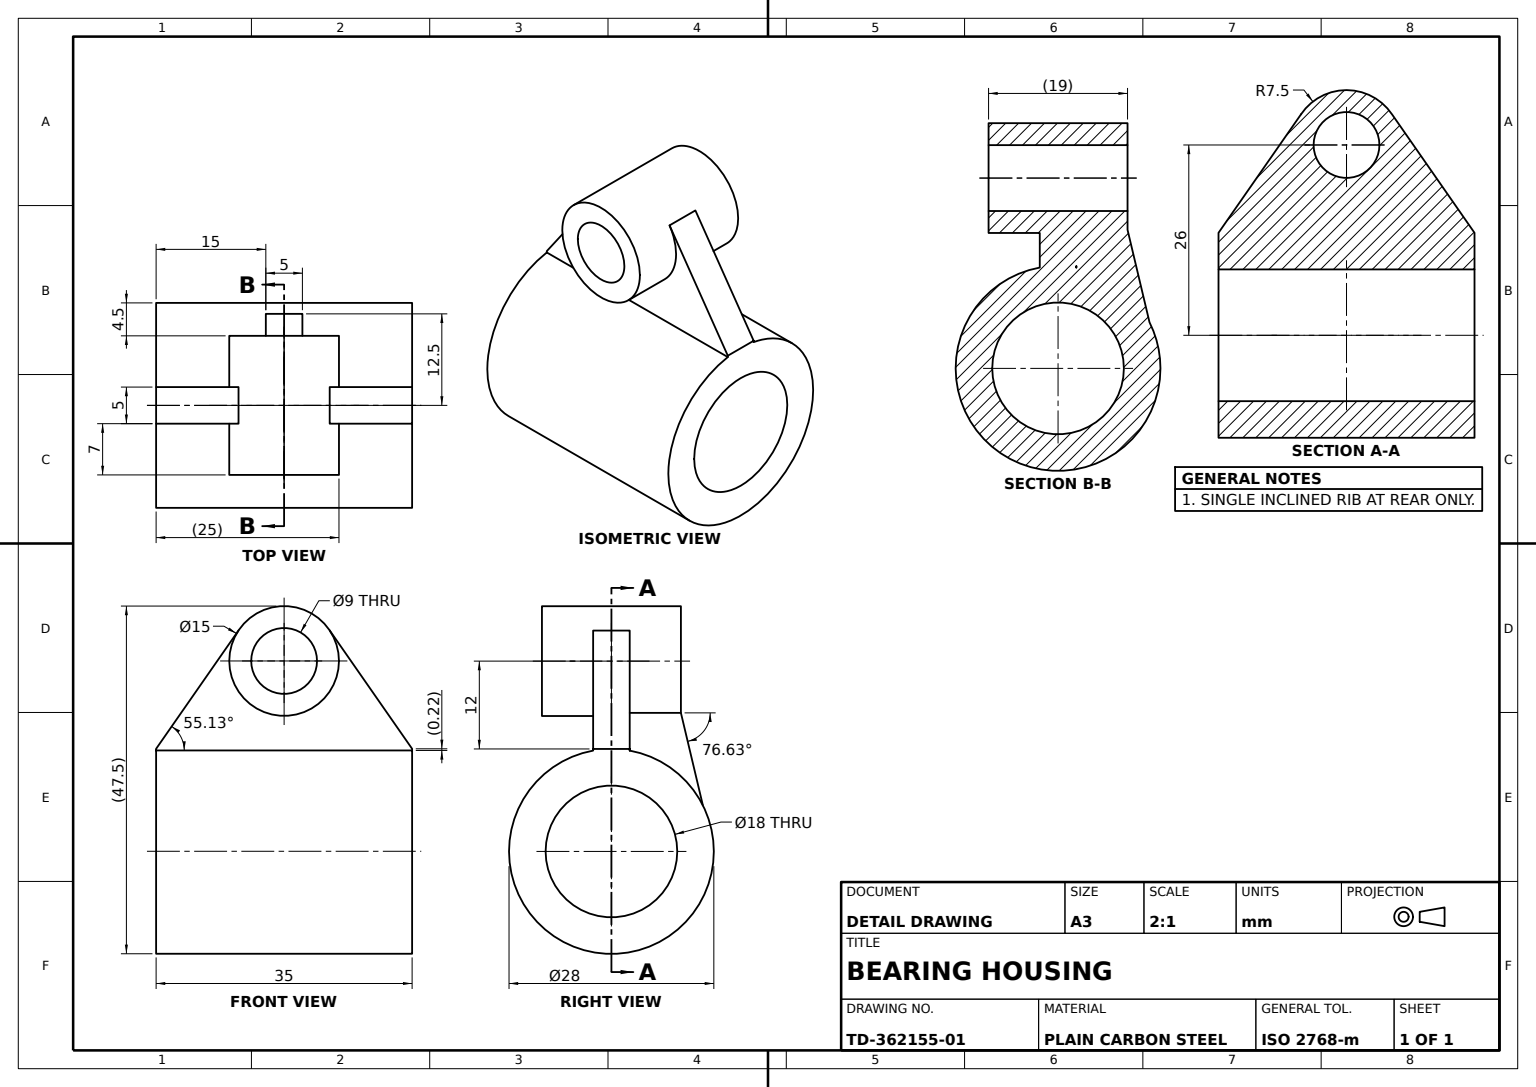
from build123d import *

# Parameters (mm, degrees)
MAIN_CYLINDER_SKETCH_R = 14
MAIN_CYLINDER_28_DEPTH = 35
MAIN_BORE_SKETCH_R     = 9
MAIN_BORE_18_DEPTH     = 35
BASE_WEB_SKETCH_R      = 7.5
BASE_WEB_DEPTH         = 2.5
SECOND_WEB_DEPTH       = 2.5
SUPPORT_RIB_DEPTH      = 5
UPPER_BOSS_A_SKETCH_R  = 7.5
UPPER_BOSS_A_15_DEPTH  = 7
UPPER_BOSS_B_SKETCH_R  = 7.5
UPPER_BOSS_B_15_DEPTH  = 7
BOSS_ARM_DEPTH         = 7
SADDLE_FILL_DEPTH      = 35
TRIM_CUT_1_DEPTH       = 15
TRIM_CUT_2_DEPTH       = 51.430645445
TRIM_CUT_2_DEPTH_BACK  = 15
TRIM_CUT_3_DEPTH       = 15
UPPER_BORE_SKETCH_R    = 4.5
UPPER_BORE_9_DEPTH     = 50
CYLINDER_SKIN_28_DEPTH = 35


with BuildPart() as part:
    # Main Cylinder Sketch → Main Cylinder Ø28 (new body)
    with BuildSketch(Plane.XY):
        Circle(MAIN_CYLINDER_SKETCH_R)
    extrude(amount=-MAIN_CYLINDER_28_DEPTH)

    # Main Bore Sketch → Main Bore Ø18 (cut)
    with BuildSketch(Plane.XY):
        Circle(MAIN_BORE_SKETCH_R)
    extrude(amount=-MAIN_BORE_18_DEPTH, mode=Mode.SUBTRACT)



with BuildPart() as body_2:
    # Base Web Sketch → Base Web (new body)
    with BuildSketch(Plane(origin=(0, 0, 0), x_dir=(0, 0, -1), z_dir=(1, 0, 0))):
        with Locations((17.5, 26)):
            Circle(BASE_WEB_SKETCH_R)
        with BuildLine():
            Line((35, 14), (25, 26))
            ThreePointArc((25, 26), (17.5, 18.5), (10, 26))
            Line((10, 26), (0, 14))
            Line((0, 14), (35, 14))
        make_face()
    extrude(amount=-BASE_WEB_DEPTH)

    # Second Web Sketch → Second Web (add)
    with BuildSketch(Plane(origin=(0, 0, 0), x_dir=(0, 0, -1), z_dir=(1, 0, 0))):
        with BuildLine():
            ThreePointArc((25, 26), (17.5, 33.5), (10, 26))
            ThreePointArc((10, 26), (17.5, 18.5), (25, 26))
        make_face()
        with BuildLine():
            Line((10, 26), (0, 14))
            Line((0, 14), (35, 14))
            Line((35, 14), (25, 26))
            ThreePointArc((25, 26), (17.5, 18.5), (10, 26))
        make_face()
    extrude(amount=SECOND_WEB_DEPTH)

    # Support Rib Sketch → Support Rib (add)
    with BuildSketch(Plane(origin=(2.5, 0, 0), x_dir=(0, 0, -1), z_dir=(1, 0, 0))):
        with BuildLine():
            Line((11.267674623, 30.172303968), (0, 14))
            Line((0, 14), (10, 26))
            ThreePointArc((10, 26), (10.323913311, 28.180316454), (11.267674623, 30.172303968))
        make_face()
        with BuildLine():
            Line((25, 26), (35, 14))
            Line((35, 14), (23.732325377, 30.172303968))
            ThreePointArc((23.732325377, 30.172303968), (24.676086689, 28.180316454), (25, 26))
        make_face()
    extrude(amount=-SUPPORT_RIB_DEPTH)

    # Upper Boss A Sketch → Upper Boss A Ø15 (add)
    with BuildSketch(Plane(origin=(2.5, 0, 0), x_dir=(0, 0, -1), z_dir=(1, 0, 0))):
        with Locations((17.5, 26)):
            Circle(UPPER_BOSS_A_SKETCH_R)
    extrude(amount=UPPER_BOSS_A_15_DEPTH)

    # Upper Boss B Sketch → Upper Boss B Ø15 (add)
    with BuildSketch(Plane.ZY.offset(2.5)):
        with Locations(Location((-17.5, 26, 0), (0, 0, 180))):
            Circle(UPPER_BOSS_B_SKETCH_R)
    extrude(amount=UPPER_BOSS_B_15_DEPTH)

    # Upper Bore Sketch → Upper Bore Ø9 (cut)
    with BuildSketch(Plane(origin=(9.5, 0, 0), x_dir=(0, 0, -1), z_dir=(1, 0, 0))):
        with Locations((17.5, 26)):
            Circle(UPPER_BORE_SKETCH_R)
    extrude(amount=-UPPER_BORE_9_DEPTH, mode=Mode.SUBTRACT)


with BuildPart() as body_3:
    # Boss Arm Sketch → Boss Arm (new body)
    with BuildSketch(Plane(origin=(9.5, 0, 0), x_dir=(0, 0, -1), z_dir=(1, 0, 0))):
        with BuildLine():
            Line((15, 18.5), (15, 18.928932188))
            ThreePointArc((15, 18.928932188), (17.5, 18.5), (20, 18.928932188))
            Line((20, 18.928932188), (20, 0))
            Line((20, 0), (15, 0))
            Line((15, 0), (15, 18.5))
        make_face()
    extrude(amount=-BOSS_ARM_DEPTH)

    # Trim Cut 3 Sketch → Trim Cut 3 (cut)
    with BuildSketch(Plane.XY.offset(-15)):
        with BuildLine():
            Line((2.5, 0), (9, 0))
            ThreePointArc((9, 0), (7.193747285, 5.408326913), (2.5, 8.645808233))
            Line((2.5, 8.645808233), (2.5, 0))
        make_face()
    extrude(amount=-TRIM_CUT_3_DEPTH, mode=Mode.SUBTRACT)


with BuildPart() as body_4:
    # Saddle Fill Sketch → Saddle Fill (new body)
    with BuildSketch(Plane.XY):
        with BuildLine():
            Line((9.5, 18.928932188), (12.50219707, 6.300402243))
            ThreePointArc((12.50219707, 6.300402243), (8.380560683, 11.214553163), (2.5, 13.774977314))
            Line((2.5, 13.774977314), (2.5, 18.928932188))
            Line((2.5, 18.928932188), (9.5, 18.928932188))
        make_face()
    extrude(amount=-SADDLE_FILL_DEPTH)

    # Trim Cut 1 Sketch → Trim Cut 1 (cut)
    with BuildSketch(Plane.XY):
        with BuildLine():
            Line((2.5, 18.928932188), (9.5, 18.928932188))
            Line((9.5, 18.928932188), (12.50219707, 6.300402243))
            ThreePointArc((12.50219707, 6.300402243), (8.380560683, 11.214553163), (2.5, 13.774977314))
            Line((2.5, 13.774977314), (2.5, 18.928932188))
        make_face()
    extrude(amount=-TRIM_CUT_1_DEPTH, mode=Mode.SUBTRACT)

    # Trim Cut 2 Sketch → Trim Cut 2 (cut, two sides: drawn at the far end of the back side and taken through both)
    with BuildSketch(Plane(origin=(0, 0, -35), x_dir=(-1, 0, 0), z_dir=(0, 0, -1)).offset(-TRIM_CUT_2_DEPTH_BACK)):
        with BuildLine():
            Line((-2.5, 18.928932188), (-9.5, 18.928932188))
            Line((-9.5, 18.928932188), (-12.50219707, 6.300402243))
            ThreePointArc((-12.50219707, 6.300402243), (-8.380560683, 11.214553163), (-2.5, 13.774977314))
            Line((-2.5, 13.774977314), (-2.5, 18.928932188))
        make_face()
    extrude(amount=TRIM_CUT_2_DEPTH + TRIM_CUT_2_DEPTH_BACK, mode=Mode.SUBTRACT)


with BuildPart() as part_1:
    add(part.part)

    add(body_2.part)  # Cylinder Skin Ø28 merges body 2

    add(body_3.part)  # Cylinder Skin Ø28 merges body 3

    add(body_4.part)  # Cylinder Skin Ø28 merges body 4
    # Cylinder Skin Sketch → Cylinder Skin Ø28 (add)
    with BuildSketch(Plane.XY):
        with BuildLine():
            Line((2.5, 14), (1.6e-08, 14))
            ThreePointArc((1.6e-08, 14), (1.252779423, 13.94383533), (2.495507125, 13.775791962))
            Line((2.495507125, 13.775791962), (2.5, 14))
        make_face()
        with BuildLine():
            Line((1.6e-08, 14), (-2.5, 14))
            Line((-2.5, 14), (-2.5, 13.774977314))
            ThreePointArc((-2.5, 13.774977314), (-1.255053299, 13.943630848), (1.6e-08, 14))
        make_face()
    extrude(amount=-CYLINDER_SKIN_28_DEPTH)


solid = part_1.part
